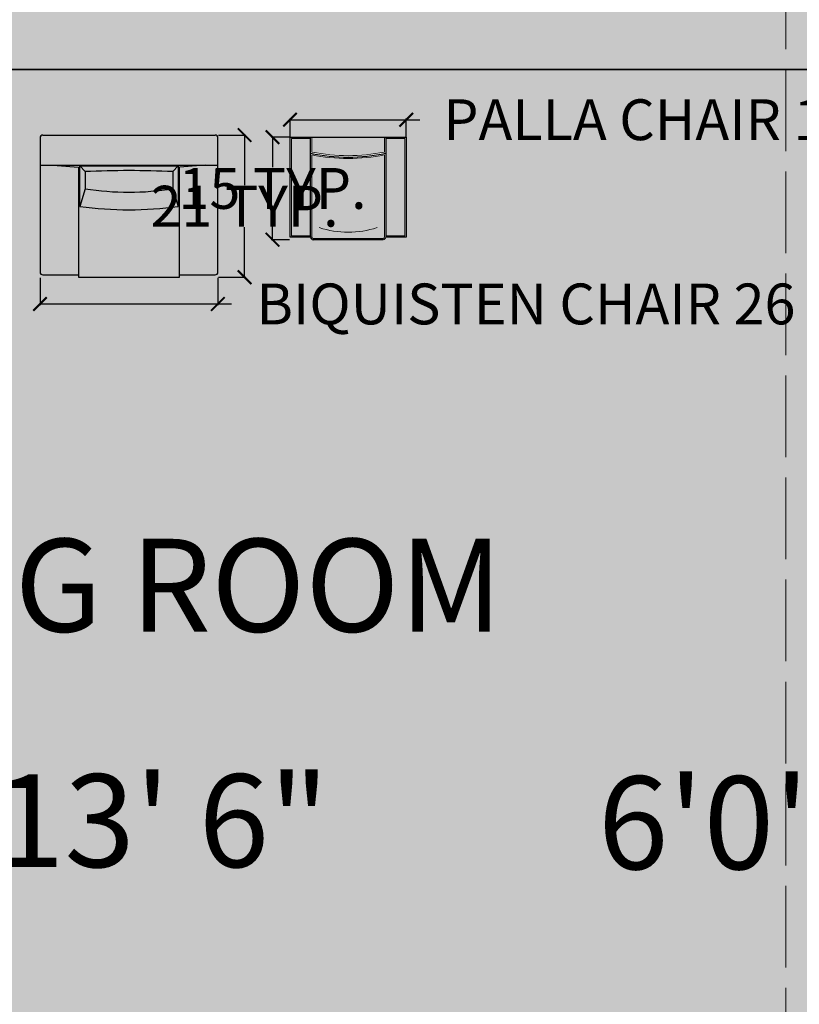
# Model space of a CAD drawing. Units: inches. Extents: x 1704 to 6393, y -157 to 1172.
# Tile 22 of 122: x 2161 to 2275, y 227 to 372. Entities that reach past the tile are written whole.
import ezdxf

# ---------------------------------------------------------------- set-up
doc = ezdxf.new("R2010")
doc.units = ezdxf.units.IN
doc.header["$MEASUREMENT"] = 0
doc.linetypes.add('ACAD_ISO02W100', pattern=[15, 12, -3])
for name, color, linetype, lineweight in [('A-ANNO-DIMS', 7, 'Continuous', 13), ('A-AREA-IDEN', 7, 'Continuous', 18), ('A-FURN', 8, 'Continuous', 18), ('A-WALL-OVHD', 8, 'ACAD_ISO02W100', 13), ('A-WALL-PATT', 7, 'Continuous', 13), ('estofado', 7, 'Continuous', 25), ('hachura', 252, 'Continuous', 5), ('moveis', 254, 'Continuous', 5), ('WALLS', 7, 'Continuous', 35)]:
    doc.layers.add(name, color=color, linetype=linetype, lineweight=lineweight)
doc.layers.add('A-FLOR-PATT', color=7, linetype='Continuous', lineweight=13, true_color=0xf2f2f2)
doc.layers.add('MESA', color=7, linetype='Continuous')
doc.styles.get("Standard").update_dxf_attribs({"font": 'arial.ttf'})
doc.dimstyles.get("Standard").update_dxf_attribs({"dimtxt": 6, "dimasz": 2, "dimexe": 0.18, "dimexo": 0.0625, "dimgap": 0.09, "dimtad": 0, "dimtih": 1, "dimtoh": 1, "dimdec": 1, "dimzin": 0, "dimdsep": 46, "dimlunit": 3, "dimtxsty": 'Standard', "dimblk": 'ARCHTICK', "dimcen": 0.09, "dimadec": 0, "dimazin": 0, "dimtfac": 1, "dimtdec": 1, "dimtofl": 0, "dimtmove": 0, "dimatfit": 3, "dimfxl": 1, "dimtolj": 1, "dimtzin": 0, "dimarcsym": 0})

# ---------------------------------------------------------------- blocks, each defined once
blk = doc.blocks.new('Poltrona Palla')
at = {"layer": 'hachura'}
h = blk.add_hatch(color=256, dxfattribs=at)
h.dxf.hatch_style = 1
h.set_gradient(color1=(73, 95, 131), color2=(46, 60, 82), one_color=1, tint=0.25, name='INVCYLINDER')
h.paths.add_polyline_path([(0.265, 0), (-0.265, 0), (-0.265, -0.1089, 0.101458), (0.265, -0.1089)])
h = blk.add_hatch(color=256, dxfattribs=at)
h.dxf.hatch_style = 1
h.set_gradient(color1=(73, 95, 131), color2=(35, 45, 62), one_color=1, tint=0.19)
h.paths.add_polyline_path([(-0.275, -0.01), (-0.415, -0.01), (-0.415, -0.7213), (-0.275, -0.7213)])
h = blk.add_hatch(color=256, dxfattribs=at)
h.dxf.hatch_style = 1
h.set_gradient(color1=(73, 95, 131), color2=(35, 45, 62), one_color=1, tint=0.19)
h.paths.add_polyline_path([(0.415, -0.01), (0.275, -0.01), (0.275, -0.7213), (0.415, -0.7213)])
h = blk.add_hatch(color=256, dxfattribs=at)
h.dxf.hatch_style = 1
h.set_gradient(color1=(73, 95, 131), color2=(35, 45, 62), one_color=1, tint=0.19, name='INVCURVED')
h.paths.add_polyline_path([(0.265, -0.1293, -0.099912), (-0.265, -0.1293), (-0.265, -0.73, 0.414214), (-0.255, -0.74), (0.255, -0.74, 0.414214), (0.265, -0.73)])
at = {"layer": 'MESA'}
for p, q in [((-0.425, 0), (0.425, 0)), ((-0.425, -0.7313), (-0.425, 0)), ((-0.275, -0.73), (-0.275, 0)), ((0.275, 0), (0.275, -0.73)), ((0.425, 0), (0.425, -0.7313)), ((-0.275, -0.7313), (-0.425, -0.7313)), ((0.255, -0.75), (-0.255, -0.75)), ((0.425, -0.7313), (0.275, -0.7313))]:
    blk.add_line(p, q, dxfattribs=at)
for centre, radius, start, end in [((0, 1.1836), 1.3294, 258.06163, 281.93837), ((-0.255, -0.73), 0.02, 180, 270)]:
    blk.add_arc(centre, radius, start, end, dxfattribs=at)
at = {"layer": 'moveis', "ltscale": 0.05}
for p, q in [((-0.265, -0.1089), (-0.265, 0)), ((0.265, 0), (0.265, -0.1089)), ((-0.415, -0.01), (-0.275, -0.01)), ((-0.415, -0.7213), (-0.415, -0.01)), ((0.275, -0.01), (0.415, -0.01)), ((0.415, -0.01), (0.415, -0.7213)), ((-0.265, -0.73), (-0.265, -0.1293)), ((0.265, -0.1293), (0.265, -0.73)), ((-0.275, -0.7213), (-0.415, -0.7213)), ((0.255, -0.74), (-0.255, -0.74)), ((0.415, -0.7213), (0.275, -0.7213))]:
    blk.add_line(p, q, dxfattribs=at)
for centre, radius, start, end in [((0, 1.1836), 1.3194, 258.41345, 281.58655), ((0, 1.1836), 1.3394, 258.5888, 281.4112), ((0, -0.0151), 0.6799, 251.92101, 288.07899), ((-0.255, -0.73), 0.01, 180, 270), ((0.255, -0.73), 0.01, 270, 360), ((0.255, -0.73), 0.02, 270, 360)]:
    blk.add_arc(centre, radius, start, end, dxfattribs=at)
blk = doc.blocks.new('poltrona biquisten 2')
at = {"layer": 'estofado', "ltscale": 0.5}
h = blk.add_hatch(color=256, dxfattribs=at)
h.dxf.hatch_style = 1
h.set_gradient(color1=(165, 192, 175), color2=(222, 232, 226), one_color=1, tint=0.89, name='INVCURVED')
h.paths.add_polyline_path([(0.65, 1.02, 0.414214), (0.63, 1.04), (-0.63, 1.04, 0.414214), (-0.65, 1.02), (-0.65, 0.82), (0.65, 0.82)])
h = blk.add_hatch(color=256, dxfattribs=at)
h.dxf.hatch_style = 1
h.set_gradient(color1=(165, 192, 175), color2=(222, 232, 226), one_color=1, tint=0.89)
h.paths.add_polyline_path([(-0.37, 0.8064), (-0.5562, 0.82), (-0.65, 0.82), (-0.65, 0.0379, 0.414214), (-0.63, 0.0179), (-0.37, 0.0179)])
h = blk.add_hatch(color=256, dxfattribs=at)
h.dxf.hatch_style = 1
h.set_gradient(color1=(165, 192, 175), color2=(222, 232, 226), one_color=1, tint=0.89, name='INVCURVED')
h.paths.add_polyline_path([(0.37, 0.8064), (0.5562, 0.82), (-0.5562, 0.82), (-0.37, 0.8064), (-0.37, 0), (0.37, 0)])
h.paths.add_polyline_path([(-0.3585, 0.5186), (-0.3585, 0.8144), (0.3585, 0.8144), (0.3585, 0.5186, -0.068679)], flags=16)
h.paths.add_polyline_path([(-0.3207, 0.6475), (-0.3207, 0.7727, -0.023546), (0.3207, 0.7727), (0.3207, 0.6475, -0.077277)], flags=0)
h = blk.add_hatch(color=256, dxfattribs=at)
h.dxf.hatch_style = 1
h.set_gradient(color1=(165, 192, 175), color2=(222, 232, 226), one_color=1, tint=0.89, name='CYLINDER')
h.paths.add_polyline_path([(0.3585, 0.8144), (-0.3585, 0.8144), (-0.3207, 0.7727, -0.023546), (0.3207, 0.7727)])
h = blk.add_hatch(color=256, dxfattribs=at)
h.dxf.hatch_style = 1
h.set_gradient(color1=(165, 192, 175), color2=(222, 232, 226), one_color=1, tint=0.89, name='CYLINDER')
h.paths.add_polyline_path([(-0.3207, 0.7727), (-0.3585, 0.8144), (-0.3585, 0.5186), (-0.3207, 0.6475)])
h.paths.add_polyline_path([(0.3585, 0.8144), (0.3207, 0.7727), (0.3207, 0.6475), (0.3585, 0.5186)])
h.paths.add_polyline_path([(0.3207, 0.6475, -0.077277), (-0.3207, 0.6475), (-0.3585, 0.5186, 0.068679), (0.3585, 0.5186)])
h = blk.add_hatch(color=256, dxfattribs=at)
h.dxf.hatch_style = 1
h.set_gradient(color1=(165, 192, 175), color2=(222, 232, 226), one_color=1, tint=0.89)
h.paths.add_polyline_path([(0.65, 0.82), (0.5562, 0.82), (0.37, 0.8064), (0.37, 0.0179), (0.63, 0.0179, 0.414214), (0.65, 0.0379)])
h = blk.add_hatch(color=256, dxfattribs=at)
h.dxf.hatch_style = 1
h.set_gradient(color1=(165, 192, 175), color2=(222, 232, 226), one_color=1, tint=0.89, name='INVCURVED')
h.paths.add_polyline_path([(0.3207, 0.7727, 0.023546), (-0.3207, 0.7727), (-0.3207, 0.6475, 0.077277), (0.3207, 0.6475)])
for p, q in [((-0.65, 1.02), (-0.65, 0.0379)), ((-0.63, 1.04), (0.63, 1.04)), ((0.65, 0.0379), (0.65, 1.02)), ((-0.65, 0.82), (0.65, 0.82)), ((-0.5562, 0.82), (-0.37, 0.8064)), ((-0.37, 0.8064), (-0.37, 0)), ((-0.3585, 0.8144), (-0.3207, 0.7727)), ((0.3585, 0.8144), (0.3207, 0.7727)), ((0.5562, 0.82), (0.37, 0.8064)), ((0.37, 0), (0.37, 0.8064)), ((-0.3207, 0.7727), (-0.3207, 0.6475)), ((0.3207, 0.7727), (0.3207, 0.6475)), ((-0.3207, 0.6475), (-0.3585, 0.5186)), ((0.3207, 0.6475), (0.3585, 0.5186)), ((-0.63, 0.0179), (-0.37, 0.0179)), ((-0.37, 0), (0.37, 0)), ((0.37, 0.0179), (0.63, 0.0179))]:
    blk.add_line(p, q, dxfattribs=at)
blk.add_lwpolyline([(-0.3585, 0.5186), (-0.3585, 0.8144), (0.3585, 0.8144), (0.3585, 0.5186)], dxfattribs=at)
for centre, radius, start, end in [((-0.63, 1.02), 0.02, 90, 180), ((0.63, 1.02), 0.02, 0, 90), ((0, -6.0334), 6.8136, 87.3023, 92.6977), ((0, 2.7101), 2.0874, 261.16232, 278.83768), ((0, 3.1159), 2.6219, 262.14225, 277.85775), ((-0.63, 0.0379), 0.02, 180, 270), ((0.63, 0.0379), 0.02, 270, 0)]:
    blk.add_arc(centre, radius, start, end, dxfattribs=at)
blk = doc.blocks.new('_ArchTick')
at = {"color": 0, "linetype": 'ByBlock', "const_width": 0.15}
blk.add_lwpolyline([(-0.5, -0.5), (0.5, 0.5)], dxfattribs=at)
blk = doc.blocks.new('*D58')
at = {"layer": 'A-ANNO-DIMS', "color": 0, "lineweight": -2, "transparency": 16777216}
for p, q in [((2200.54, 354.32), (2200.54, 357)), ((2200.54, 356.82), (2217.62, 356.82)), ((2217.62, 354.32), (2217.62, 357)), ((2217.62, 356.82), (2219.62, 356.82))]:
    blk.add_line(p, q, dxfattribs=at)
at = {"layer": 'Defpoints', "color": 0, "lineweight": -3, "transparency": 16777216}
for p in [(2217.62, 356.82), (2200.54, 354.26), (2217.62, 354.26)]:
    blk.add_point(p, dxfattribs=at)
at = {"layer": 'A-ANNO-DIMS', "color": 0, "lineweight": -2, "transparency": 16777216, "xscale": 2, "yscale": 2, "zscale": 2, "rotation": 180}
blk.add_blockref('_ArchTick', (2200.54, 356.82), dxfattribs=at)
at = {"layer": 'A-ANNO-DIMS', "color": 0, "lineweight": -2, "transparency": 16777216, "xscale": 2, "yscale": 2, "zscale": 2}
blk.add_blockref('_ArchTick', (2217.62, 356.82), dxfattribs=at)
at = {"layer": 'A-ANNO-DIMS', "color": 0, "transparency": 16777216, "insert": (2262.58, 356.82), "char_height": 6, "attachment_point": 5}
blk.add_mtext('\\A1;PALLA CHAIR 17 TYP.', dxfattribs=at)
blk = doc.blocks.new('*D59')
at = {"layer": 'A-ANNO-DIMS', "color": 0, "lineweight": -2, "transparency": 16777216}
for p, q in [((2200.47, 354.26), (2197.79, 354.26)), ((2197.97, 354.26), (2197.97, 349.87)), ((2197.97, 339.18), (2197.97, 343.57)), ((2200.47, 339.18), (2197.79, 339.18))]:
    blk.add_line(p, q, dxfattribs=at)
at = {"layer": 'Defpoints', "color": 0, "lineweight": -3, "transparency": 16777216}
for p in [(2197.97, 354.26), (2200.54, 354.26), (2200.54, 339.18)]:
    blk.add_point(p, dxfattribs=at)
at = {"layer": 'A-ANNO-DIMS', "color": 0, "lineweight": -2, "transparency": 16777216, "xscale": 2, "yscale": 2, "zscale": 2}
for p, rotation in [((2197.97, 354.26), 90), ((2197.97, 339.18), 270)]:
    blk.add_blockref('_ArchTick', p, dxfattribs=dict(at, rotation=rotation))
at = {"layer": 'A-ANNO-DIMS', "color": 0, "transparency": 16777216, "insert": (2197.97, 346.72), "char_height": 6, "attachment_point": 5}
blk.add_mtext('\\A1;15 TYP.', dxfattribs=at)
blk = doc.blocks.new('*D62')
at = {"layer": 'A-ANNO-DIMS', "color": 0, "lineweight": -2, "transparency": 16777216}
for p, q in [((2163.81, 333.6), (2163.81, 329.56)), ((2189.94, 333.6), (2189.94, 329.56)), ((2163.81, 329.74), (2189.94, 329.74)), ((2189.94, 329.74), (2191.94, 329.74))]:
    blk.add_line(p, q, dxfattribs=at)
at = {"layer": 'Defpoints', "color": 0, "lineweight": -3, "transparency": 16777216}
for p in [(2163.81, 333.66), (2189.94, 333.66), (2189.94, 329.74)]:
    blk.add_point(p, dxfattribs=at)
at = {"layer": 'A-ANNO-DIMS', "color": 0, "lineweight": -2, "transparency": 16777216, "xscale": 2, "yscale": 2, "zscale": 2, "rotation": 180}
blk.add_blockref('_ArchTick', (2163.81, 329.74), dxfattribs=at)
at = {"layer": 'A-ANNO-DIMS', "color": 0, "lineweight": -2, "transparency": 16777216, "xscale": 2, "yscale": 2, "zscale": 2}
blk.add_blockref('_ArchTick', (2189.94, 329.74), dxfattribs=at)
at = {"layer": 'A-ANNO-DIMS', "color": 0, "transparency": 16777216, "insert": (2244.46, 329.74), "char_height": 6, "attachment_point": 5}
blk.add_mtext('\\A1;BIQUISTEN CHAIR 26 TYP.', dxfattribs=at)
blk = doc.blocks.new('*D63')
at = {"layer": 'A-ANNO-DIMS', "color": 0, "lineweight": -2, "transparency": 16777216}
for p, q in [((2190.01, 354.56), (2194.04, 354.56)), ((2193.86, 354.56), (2193.86, 347.21)), ((2193.86, 333.66), (2193.86, 341.01)), ((2190.01, 333.66), (2194.04, 333.66))]:
    blk.add_line(p, q, dxfattribs=at)
at = {"layer": 'Defpoints', "color": 0, "lineweight": -3, "transparency": 16777216}
for p in [(2189.94, 354.56), (2193.86, 354.56), (2189.94, 333.66)]:
    blk.add_point(p, dxfattribs=at)
at = {"layer": 'A-ANNO-DIMS', "color": 0, "lineweight": -2, "transparency": 16777216, "xscale": 2, "yscale": 2, "zscale": 2}
for p, rotation in [((2193.86, 354.56), 90), ((2193.86, 333.66), 270)]:
    blk.add_blockref('_ArchTick', p, dxfattribs=dict(at, rotation=rotation))
at = {"layer": 'A-ANNO-DIMS', "color": 0, "transparency": 16777216, "insert": (2193.86, 344.11), "char_height": 6, "attachment_point": 5}
blk.add_mtext('\\A1;21 TYP.', dxfattribs=at)
blk = doc.blocks.new('*D93')
at = {"layer": 'A-ANNO-DIMS', "color": 0, "lineweight": -2, "transparency": 16777216}
for p, q in [((2605.29, 895.21), (1829.7, 895.21)), ((1829.88, 895.21), (1829.88, 495.87)), ((1829.88, 90.21), (1829.88, 489.56)), ((2605.29, 90.21), (1829.7, 90.21))]:
    blk.add_line(p, q, dxfattribs=at)
at = {"layer": 'Defpoints', "color": 0, "lineweight": -3, "transparency": 16777216}
for p in [(2605.35, 895.21), (1829.88, 90.21), (2605.35, 90.21)]:
    blk.add_point(p, dxfattribs=at)
at = {"layer": 'A-ANNO-DIMS', "color": 0, "lineweight": -2, "transparency": 16777216, "xscale": 2, "yscale": 2, "zscale": 2}
for p, rotation in [((1829.88, 895.21), 90), ((1829.88, 90.21), 270)]:
    blk.add_blockref('_ArchTick', p, dxfattribs=dict(at, rotation=rotation))
at = {"layer": 'A-ANNO-DIMS', "color": 0, "transparency": 16777216, "insert": (1829.88, 492.71), "char_height": 6, "attachment_point": 5}
blk.add_mtext('\\A1;805', dxfattribs=at)

msp = doc.modelspace()

# ---------------------------------------------------------------- hatches: boundary and pattern name
at = {"layer": 'A-FLOR-PATT', "transparency": 33554528}
h = msp.add_hatch(color=256, dxfattribs=at)
h.dxf.hatch_style = 1
h.paths.add_polyline_path([(2273.349, 538.213), (2081.349, 538.213), (2081.349, 372.213), (2273.349, 372.213)])
h.paths.add_polyline_path([(2189.542, 505.951), (2184.316, 505.951), (2184.316, 505.591), (2169.442, 505.591), (2169.442, 505.951), (2164.216, 505.951, -0.4142136), (2163.814, 506.353), (2163.814, 526.093, -0.4142136), (2164.216, 526.495), (2189.542, 526.495, -0.4142136), (2189.944, 526.093), (2189.944, 506.353, -0.4142136)], flags=16)
h.paths.add_polyline_path([(2200.535, 511.491), (2200.535, 526.191), (2217.621, 526.191), (2217.621, 511.491), (2214.605, 511.491, -0.3946213), (2214.203, 511.116), (2203.952, 511.116, -0.3946213), (2203.551, 511.491)], flags=16)
h.paths.add_polyline_path([(2200.736, 511.692), (2200.736, 525.99), (2203.55, 525.99), (2203.55, 523.838, 0.1045605), (2214.605, 523.838), (2214.605, 525.99), (2217.42, 525.99), (2217.42, 511.692), (2214.605, 511.692), (2214.605, 523.838, -0.1045605), (2203.55, 523.838), (2203.55, 511.692)], flags=0)
h.paths.add_polyline_path([(2203.952, 511.317, -0.4142136), (2203.751, 511.518), (2203.751, 523.591, 0.099912), (2214.404, 523.591), (2214.404, 511.518, -0.4142136), (2214.203, 511.317)], flags=0)
h.paths.add_polyline_path([(2184.084, 516.015, -0.0686795), (2169.674, 516.015), (2169.674, 522.073), (2184.084, 522.073)], flags=0)
h.paths.add_polyline_path([(2183.325, 518.606, -0.0772766), (2170.433, 518.606), (2170.433, 521.123, -0.0235462), (2183.325, 521.123)], flags=0)
h.paths.add_polyline_path([(2135.029, 507.225, -0.1405189), (2135.191, 507.834, -0.0513838), (2135.029, 507.797)], flags=16)
h.paths.add_polyline_path([(2146.318, 498.997, -0.0311848), (2144.279, 499.202, -0.1719602), (2141.865, 499.263, -0.2234326), (2139.482, 499.263, -0.1719602), (2137.068, 499.202, -0.0311848), (2135.029, 498.997, -0.066975), (2135.029, 505.313, -0.0276914), (2136.841, 505.144), (2136.841, 506.777), (2136.576, 506.777), (2136.576, 507.371, 0.039911), (2145.741, 507.448, 0.2546956), (2146.318, 507.225), (2146.318, 507.269, 0.1305786), (2146.156, 507.834, -0.0704067), (2145.953, 507.935, -0.011584), (2145.714, 508.002, -0.2546956), (2145.137, 507.779, -0.2546956), (2145.361, 508.355, -0.0259693), (2145.107, 516.407, -0.0070422), (2144.025, 516.297, -0.1828112), (2142.939, 516.218, -0.2042746), (2142.015, 516.175, -0.1805419), (2139.348, 516.174, -0.0000184), (2139.345, 516.174, -0.2035615), (2138.425, 516.217, -0.0000237), (2138.421, 516.217, -0.1818152), (2137.34, 516.296, -0.0071635), (2136.24, 516.407, 0.007166), (2136.162, 518.63, 0.314303), (2135.854, 518.974, -0.1253469), (2135.537, 518.935, -0.2546956), (2135.76, 519.512, -0.0162662), (2135.67, 519.849, -0.296972), (2135.535, 520.8, -0.227702), (2135.464, 521.698, 0.1283977), (2132.757, 521.718), (2132.757, 525.785, -0.4142136), (2133.331, 526.359), (2148.015, 526.359, -0.4142136), (2148.589, 525.785), (2148.589, 521.718, -0.0118936), (2148.835, 521.65, -0.2546956), (2149.412, 521.873, -0.2546956), (2149.188, 521.296, -0.0417628), (2149.188, 508.355, -0.2546956), (2149.412, 507.779, -0.2546956), (2148.835, 508.002, -0.011584), (2148.596, 507.935, -0.2124435), (2147.949, 507.813, -0.2363999), (2147.423, 507.772, -0.3143526), (2147.126, 507.772, -0.2363999), (2146.6, 507.813, -0.0879275), (2146.318, 507.797), (2146.318, 507.225, -0.2546956), (2145.741, 507.448, -0.0042329), (2144.771, 507.371), (2144.771, 506.777), (2144.506, 506.777), (2144.506, 505.144, -0.0276914), (2146.318, 505.313, -0.066975)], flags=16)
h.paths.add_polyline_path([(2141.865, 505.047, 0.2234326), (2139.482, 505.047, 0.1738145), (2137.043, 505.1), (2137.043, 506.317), (2137.335, 506.317), (2137.335, 505.184, -0.1522072), (2139.482, 505.047, -0.2234326), (2141.865, 505.047, -0.1522072), (2144.011, 505.184), (2144.011, 506.317), (2144.304, 506.317), (2144.304, 505.1, 0.1738145)], flags=0)
h.paths.add_polyline_path([(2145.233, 522.986, 0.0079197), (2144.017, 523.111, 0.1826165), (2142.931, 523.19, 0.2042746), (2142.008, 523.233, 0.1806536), (2139.339, 523.233, 0.2042746), (2138.415, 523.19, 0.1826165), (2137.33, 523.111, 0.0079197), (2136.114, 522.986, 0.1967082), (2135.679, 523.212, 0.047677), (2135.755, 524.004), (2134.638, 521.852), (2134.376, 524.691, -0.2583282), (2135.029, 526.359, -0.0890464), (2135.632, 525.01, -0.1830277), (2145.715, 525.01, -0.0890464), (2146.318, 526.359, -0.2583282), (2146.971, 524.691), (2146.709, 521.852), (2145.592, 524.004, 0.047677), (2145.668, 523.212, 0.1967082)], flags=0)
h.paths.add_polyline_path([(2144.419, 519.027, -0.0368796), (2136.927, 519.027, -0.0368796)], flags=0)
h.paths.add_polyline_path([(2273.349, 629.213), (2213.349, 629.213), (2213.349, 573.213), (2213.349, 545.213), (2273.349, 545.213)])
h.paths.add_polyline_path([(2273.349, 711.213), (2207.349, 711.213), (2207.349, 709.213), (2231.349, 709.213), (2231.349, 707.213), (2207.349, 707.213), (2207.349, 631.213), (2273.349, 631.213)])
h.paths.add_polyline_path([(2273.349, 364.213), (2081.349, 364.213), (2081.349, 202.213), (2225.349, 202.213), (2229.181, 202.213), (2230.482, 202.213), (2268.215, 202.213), (2269.516, 202.213), (2273.349, 202.213)])
h.paths.add_polyline_path([(2203.551, 339.558, 0.3946213), (2203.952, 339.183), (2214.203, 339.183), (2214.203, 339.384), (2203.751, 339.384), (2203.751, 339.558)], flags=16)
h.paths.add_polyline_path([(2203.55, 351.7), (2203.55, 339.759), (2200.535, 339.759), (2200.535, 354.258), (2217.621, 354.258), (2217.621, 339.558), (2214.404, 339.558), (2214.404, 351.659, -0.101837)], flags=16)
h.paths.add_polyline_path([(2214.404, 354.057), (2214.605, 354.057), (2214.605, 354.258), (2214.404, 354.258)], flags=16)
h.paths.add_polyline_path([(2189.542, 334.018), (2184.316, 334.018), (2184.316, 333.658), (2169.442, 333.658), (2169.442, 334.018), (2164.216, 334.018, -0.4142136), (2163.814, 334.42), (2163.814, 354.161, -0.4142136), (2164.216, 354.563), (2189.542, 354.563, -0.4142136), (2189.944, 354.161), (2189.944, 334.42, -0.4142136)], flags=16)
h.paths.add_polyline_path([(2184.084, 344.083, -0.0686795), (2169.674, 344.083), (2169.674, 349.85), (2165.7, 350.14), (2188.058, 350.14), (2184.084, 349.85)], flags=0)
h.paths.add_polyline_path([(2183.325, 346.673, -0.0772766), (2170.433, 346.673), (2170.433, 349.19, -0.0235462), (2183.325, 349.19)], flags=0)
h.paths.add_polyline_path([(2134.638, 349.919), (2134.376, 352.758, -0.2583282), (2135.029, 354.426), (2133.331, 354.426, 0.4142136), (2132.757, 353.852), (2132.757, 349.785, -0.0886664)], flags=16)
h.paths.add_polyline_path([(2136.114, 351.053, -0.0079197), (2137.33, 351.178, -0.1826165), (2138.415, 351.257, -0.2042746), (2139.339, 351.3, -0.1806536), (2142.008, 351.3, -0.2042746), (2142.931, 351.257, -0.1826165), (2144.017, 351.178, -0.0079197), (2145.233, 351.053, -0.1967082), (2145.668, 351.279, -0.047677), (2145.592, 352.071, 0.1133241), (2135.755, 352.071, -0.047677), (2135.679, 351.279, -0.1967082)], flags=16)
h.paths.add_polyline_path([(2145.184, 346.697, 0.0331414), (2145.361, 336.423, 0.2546956), (2145.137, 335.846, 0.3030408), (2145.781, 336.164, 0.2903634), (2146.6, 335.88, 0.2363999), (2147.126, 335.839, -0.280712), (2147.275, 336.69, -0.280712), (2147.423, 335.839, 0.2363999), (2147.949, 335.88, 0.2903634), (2148.768, 336.164, 0.3030408), (2149.412, 335.846, 0.2546956), (2149.188, 336.423, 0.0417628), (2149.188, 349.363, 0.2546956), (2149.412, 349.94, 0.2546956), (2148.835, 349.717, 0.1405058), (2145.883, 349.765, -0.227702), (2145.812, 348.867, -0.296972), (2145.677, 347.916, -0.0162662), (2145.586, 347.579, -0.2546956), (2145.81, 347.002, -0.1253469), (2145.493, 347.041, 0.314303)], flags=16)
h.paths.add_polyline_path([(2135.029, 335.292, -0.1405189), (2135.191, 335.901, -0.1399435), (2134.747, 335.88, -0.2363999), (2134.22, 335.839, -0.3143526), (2133.924, 335.839, -0.280712), (2134.072, 336.69, -0.280712), (2134.22, 335.839, 0.2363999), (2134.747, 335.88, 0.2903634), (2135.566, 336.164, 0.3030408), (2136.209, 335.846, 0.2546956), (2135.985, 336.423, 0.0331414), (2136.162, 346.697, 0.314303), (2135.854, 347.041, -0.1253469), (2135.537, 347.002, -0.2546956), (2135.76, 347.579, -0.0162662), (2135.67, 347.916, -0.296972), (2135.535, 348.867, -0.2999866), (2135.599, 350.01, -0.0330719), (2135.76, 350.7, -0.3502076), (2135.604, 351.492), (2134.638, 349.919), (2135.604, 351.492, 0.3502076), (2135.76, 350.7, 0.0330719), (2135.599, 350.01, 0.2999866), (2135.535, 348.867, 0.296972), (2135.67, 347.916, 0.0279375), (2135.971, 347.698, 0.3576436), (2135.537, 347.002, 0.1253469), (2135.854, 347.041, -0.3555912), (2136.165, 346.637, -0.0329482), (2135.985, 336.423, -0.2546956), (2136.209, 335.846, -0.2546956), (2135.632, 336.069, -0.011584), (2135.393, 336.003, -0.1222327), (2135.029, 335.864)], flags=16)
h.paths.add_polyline_path([(2136.841, 335.42), (2136.783, 335.423), (2136.783, 334.844), (2136.841, 334.471)], flags=16)
h.paths.add_polyline_path([(2146.318, 327.064, -0.0311848), (2144.279, 327.269, -0.1719602), (2141.865, 327.33, -0.2234326), (2139.482, 327.33, -0.1719602), (2137.068, 327.269, -0.0311848), (2135.029, 327.064, -0.066975), (2135.029, 333.38, -0.0311848), (2137.068, 333.175, -0.1719602), (2139.482, 333.114, -0.2234326), (2141.865, 333.114, -0.1522072), (2144.011, 333.251), (2144.011, 334.384), (2144.304, 335.406, 0.0020345), (2144.771, 335.438), (2144.771, 334.844), (2144.506, 333.211, -0.0276914), (2146.318, 333.38, -0.066975)], flags=16)
h.paths.add_polyline_path([(2137.129, 334.384), (2137.335, 334.384), (2137.335, 333.251), (2137.129, 333.195)], flags=16)
h.paths.add_polyline_path([(2144.419, 347.094, -0.0368796), (2136.927, 347.094, -0.0368796)], flags=16)
h = msp.add_hatch(color=256, dxfattribs=at)
h.dxf.hatch_style = 1
h.paths.add_polyline_path([(2349.349, 372.213), (2277.349, 372.213), (2277.349, 364.213), (2349.349, 364.213)])
h.paths.add_polyline_path([(2277.349, 372.213), (2273.349, 372.213), (2273.349, 364.213), (2277.349, 364.213)])
h.paths.add_polyline_path([(2277.349, 364.213), (2273.349, 364.213), (2273.349, 202.213), (2277.349, 202.213)])
h.paths.add_polyline_path([(2277.349, 538.213), (2273.349, 538.213), (2273.349, 372.213), (2277.349, 372.213)])
h.paths.add_polyline_path([(2277.349, 629.213), (2273.349, 629.213), (2273.349, 545.213), (2277.349, 545.213)])
h.paths.add_polyline_path([(2277.349, 711.213), (2273.349, 711.213), (2273.349, 631.213), (2277.349, 631.213)])
h.paths.add_polyline_path([(2277.349, 631.213), (2273.349, 631.213), (2273.349, 629.213), (2277.349, 629.213)])
at = {"layer": 'A-WALL-PATT', "transparency": 33554643}
h = msp.add_hatch(color=256, dxfattribs=at)
h.dxf.hatch_style = 1
h.paths.add_polyline_path([(2167.349, 895.213), (2073.349, 895.213), (2073.349, 887.213), (2081.349, 887.213), (2167.349, 887.213)])
h.paths.add_polyline_path([(2465.349, 895.213), (2273.349, 895.213), (2273.349, 903.213), (2263.349, 903.213), (2263.349, 895.213), (2263.349, 887.213), (2325.349, 887.213), (2325.349, 863.213), (2333.349, 863.213), (2333.349, 887.213), (2465.349, 887.213)])
h.paths.add_polyline_path([(2533.349, 895.213), (2513.349, 895.213), (2513.349, 887.213), (2513.349, 861.213), (2517.349, 861.213), (2517.349, 887.213), (2533.349, 887.213)])
h.paths.add_polyline_path([(2605.349, 895.213), (2581.349, 895.213), (2581.349, 887.213), (2597.349, 887.213), (2597.349, 854.213), (2605.349, 854.213)])
h.paths.add_polyline_path([(2605.349, 752.213), (2629.349, 752.213), (2629.349, 716.213), (2605.349, 716.213), (2605.349, 712.213), (2719.349, 712.213), (2719.349, 716.213), (2631.349, 716.213), (2631.349, 754.213), (2605.349, 754.213), (2605.349, 794.213), (2597.349, 794.213), (2597.349, 787.213), (2517.349, 787.213), (2517.349, 813.213), (2513.349, 813.213), (2513.349, 783.213), (2517.349, 783.213), (2597.349, 783.213), (2597.349, 719.213), (2517.349, 719.213), (2517.349, 753.213), (2513.349, 753.213), (2513.349, 719.213), (2365.349, 719.213), (2365.349, 763.213), (2325.349, 763.213), (2325.349, 755.213), (2357.349, 755.213), (2357.349, 719.213), (2325.349, 719.213), (2325.349, 711.213), (2547.349, 711.213), (2547.349, 615.213), (2449.349, 615.213), (2449.349, 607.213), (2514.349, 607.213), (2514.349, 546.213), (2439.349, 546.213), (2425.349, 546.213), (2425.349, 607.213), (2425.349, 615.213), (2350.349, 615.213), (2350.349, 589.713), (2358.349, 589.713), (2358.349, 610.213), (2420.349, 610.213), (2420.349, 545.213), (2358.349, 545.213), (2358.349, 565.713), (2350.349, 565.713), (2350.349, 538.213), (2469.349, 538.213), (2469.349, 459.213), (2469.349, 372.213), (2423.349, 372.213), (2423.349, 364.213), (2473.349, 364.213), (2473.349, 318.213), (2477.349, 318.213), (2477.349, 364.213), (2547.349, 364.213), (2547.349, 352.213), (2549.349, 352.213), (2549.349, 364.213), (2597.349, 364.213), (2597.349, 328.213), (2549.349, 328.213), (2547.349, 328.213), (2547.349, 326.213), (2549.349, 326.213), (2597.349, 326.213), (2605.349, 326.213), (2605.349, 377.057), (2597.349, 377.057), (2597.349, 372.213), (2477.349, 372.213), (2477.349, 451.213), (2597.349, 451.213), (2605.349, 451.213), (2605.349, 459.213), (2597.349, 459.213), (2477.349, 459.213), (2477.349, 538.213), (2597.349, 538.213), (2597.349, 495.213), (2605.349, 495.213), (2605.349, 512.213), (2631.349, 512.213), (2631.349, 568.213), (2605.349, 568.213), (2605.349, 577.213), (2597.349, 577.213), (2597.349, 542.213), (2518.349, 542.213), (2518.349, 607.213), (2532.349, 607.213), (2605.349, 607.213), (2605.349, 615.213), (2597.349, 615.213), (2551.349, 615.213), (2551.349, 711.213), (2597.349, 711.213), (2597.349, 645.213), (2605.349, 645.213), (2605.349, 712.213), (2605.349, 716.213)])
h.paths.add_polyline_path([(2605.349, 566.213), (2629.349, 566.213), (2629.349, 514.213), (2605.349, 514.213)], flags=16)
h.paths.add_polyline_path([(2381.349, 372.213), (2349.349, 372.213), (2349.349, 202.213), (2337.349, 202.213), (2337.349, 194.213), (2349.349, 194.213), (2349.349, 90.213), (2349.349, 72.213), (2357.349, 72.213), (2357.349, 90.213), (2381.349, 90.213), (2381.349, 98.213), (2357.349, 98.213), (2357.349, 266.213), (2381.349, 266.213), (2381.349, 270.213), (2353.349, 270.213), (2353.349, 364.213), (2381.349, 364.213)])
h.paths.add_polyline_path([(2605.349, 302.213), (2597.349, 302.213), (2597.349, 270.213), (2477.349, 270.213), (2477.349, 294.213), (2473.349, 294.213), (2473.349, 270.213), (2423.349, 270.213), (2423.349, 266.213), (2597.349, 266.213), (2597.349, 218.213), (2605.349, 218.213)])
h.paths.add_polyline_path([(2605.349, 146.213), (2597.349, 146.213), (2597.349, 98.213), (2429.349, 98.213), (2429.349, 90.213), (2597.349, 90.213), (2597.349, 72.213), (2605.349, 72.213), (2605.349, 90.213)])
h.paths.add_polyline_path([(2225.349, 202.213), (2049.349, 202.213), (2049.349, 194.213), (2225.349, 194.213)])
h.paths.add_polyline_path([(2289.349, 202.213), (2277.349, 202.213), (2273.349, 202.213), (2269.516, 202.213), (2269.516, 194.213), (2273.349, 194.213), (2277.349, 194.213), (2289.349, 194.213)])
h.paths.add_polyline_path([(2273.349, 372.213), (2029.19, 372.213), (2029.19, 364.213), (2273.349, 364.213)])
h.paths.add_polyline_path([(2277.349, 545.213), (2213.349, 545.213), (2213.349, 573.213), (2205.349, 573.213), (2177.349, 573.213), (2177.349, 545.213), (2073.349, 545.213), (2073.349, 538.213), (2081.349, 538.213), (2277.349, 538.213)])
h.paths.add_polyline_path([(2181.349, 545.213), (2181.349, 569.213), (2205.349, 569.213), (2205.349, 545.213)], flags=16)
h.paths.add_polyline_path([(2277.349, 719.213), (2081.349, 719.213), (2073.349, 719.213), (2073.349, 711.213), (2154.575, 711.213), (2205.349, 711.213), (2205.349, 687.213), (2205.349, 629.213), (2213.349, 629.213), (2273.349, 629.213), (2273.349, 631.213), (2207.349, 631.213), (2207.349, 707.213), (2231.349, 707.213), (2231.349, 709.213), (2207.349, 709.213), (2207.349, 711.213), (2277.349, 711.213)])

# ---------------------------------------------------------------- linework, layer by layer
at = {"layer": 'A-WALL-OVHD'}
msp.add_line((2273.349, 202.213), (2273.349, 538.213), dxfattribs=at)
at = {"layer": 'WALLS'}
msp.add_line((2277.349, 364.213), (2029.19, 364.213), dxfattribs=at)

# ---------------------------------------------------------------- block references
at = {"layer": 'A-FURN', "xscale": 20.10025524054769, "yscale": 20.10025524054769, "zscale": 20.10025524054769}
for name, p in [('poltrona biquisten 2', (2176.879, 333.658)), ('Poltrona Palla', (2209.078, 354.258))]:
    msp.add_blockref(name, p, dxfattribs=at)

# ---------------------------------------------------------------- texts
at = {"layer": 'A-ANNO-DIMS'}
for s, p in [('16\' 0" X 13\' 6"', (2088.773, 246.952)), ('6\'0" X 13\'6"', (2245.77, 246.646))]:
    msp.add_text(s, height=13.6672, dxfattribs=at).set_placement(p)
at = {"layer": 'A-AREA-IDEN'}
msp.add_text('DRAWING ROOM', height=13.6672, dxfattribs=at).set_placement((2088.773, 281.553))

# ---------------------------------------------------------------- dimensions: what is measured, and where the dimension line sits
at = {"layer": 'A-ANNO-DIMS'}
dim = msp.add_linear_dim(base=(1829.878, 90.213), p1=(2605.349, 895.213), p2=(2605.349, 90.213), angle=90, dimstyle='Standard', override={"dimdec": 0, "dimlfac": 1, "dimrnd": 0, "dimzin": 0, "dimdsep": 46, "dimlunit": 2}, dxfattribs=at)
dim.commit()
dim.dimension.update_dxf_attribs({"geometry": '*D93', "text_midpoint": (1829.878, 492.713)})
for base, p1, p2, text, picture, middle in [((2217.621, 356.821), (2200.535, 354.258), (2217.621, 354.258), 'PALLA CHAIR <> TYP.', '*D58', (2262.58, 356.821)), ((2189.944, 329.739), (2163.814, 333.658), (2189.944, 333.658), 'BIQUISTEN CHAIR <> TYP.', '*D62', (2244.46, 329.739))]:
    dim = msp.add_linear_dim(base=base, p1=p1, p2=p2, text=text, dimstyle='Standard', override={"dimdec": 0, "dimlfac": 1, "dimrnd": 0, "dimzin": 0, "dimdsep": 46, "dimlunit": 2}, dxfattribs=at)
    dim.commit()
    dim.dimension.update_dxf_attribs({"geometry": picture, "text_midpoint": middle})
for base, p1, p2, picture, middle in [((2193.863, 354.563), (2189.944, 333.658), (2189.944, 354.563), '*D63', (2193.863, 344.11)), ((2197.973, 354.258), (2200.535, 339.183), (2200.535, 354.258), '*D59', (2197.973, 346.72))]:
    dim = msp.add_linear_dim(base=base, p1=p1, p2=p2, angle=90, text='<> TYP.', dimstyle='Standard', override={"dimdec": 0, "dimlfac": 1, "dimrnd": 0, "dimzin": 0, "dimdsep": 46, "dimlunit": 2}, dxfattribs=at)
    dim.commit()
    dim.dimension.update_dxf_attribs({"geometry": picture, "text_midpoint": middle})

doc.saveas('drawing.dxf')
